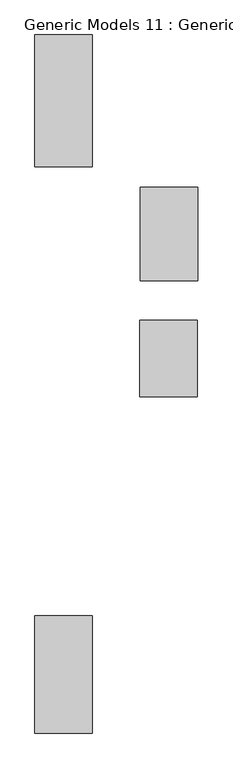
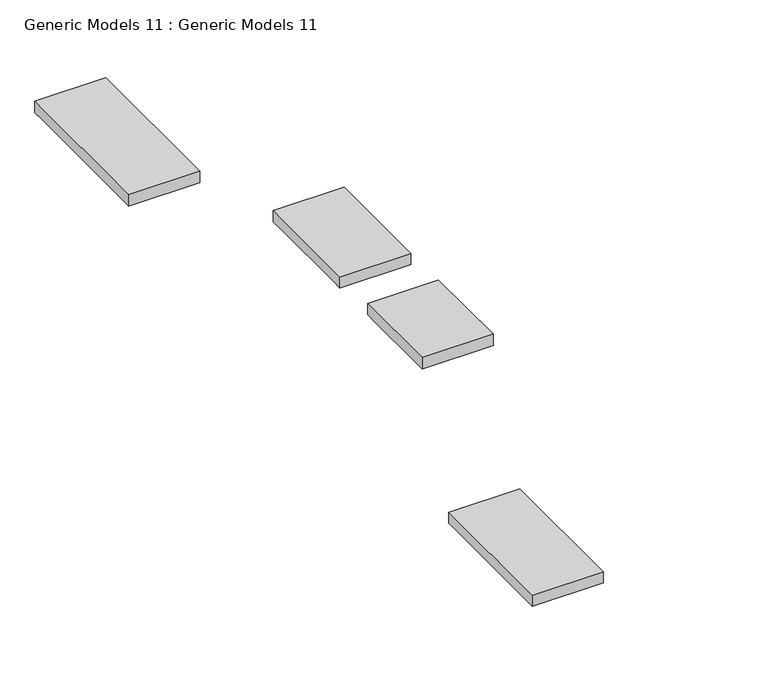
"""IFC4 building model written with IfcOpenShell, lengths in millimetres: proxy geometry, Generic Models 11 : Generic Models 11."""

from ifc_helpers import new_model, si_unit, frame, origin, place, context, project, spatial, polyline, outline, extrude, source, transform, mapped, element, save


def generic_models_11_generic_models_11_73ad1d2d(model_context):
    return source(origin(), model_context, "Body", "SweptSolid", [
        extrude(outline(polyline([(8100.454021, 5848.35), (7948.054021, 5848.35), (6385.954021, 5848.35), (6233.554021, 5848.35), (6233.554021, 6000.75), (8100.454021, 6000.75), (8100.454021, 5848.35)])), frame((-43007.0645004, 0.0, 0.0), z_axis=(1.0, 0.0, 0.0), x_axis=(0.0, 1.0, 0.0)), (0.0, 0.0, 1.0), 914.4),
        extrude(outline(polyline([(11586.604021, 5257.8), (11586.604021, 5410.2), (12805.804021, 5410.2), (12805.804021, 5257.8), (12653.404021, 5257.8), (11739.004021, 5257.8), (11586.604021, 5257.8)])), frame((-41337.0145004, 0.0, 0.0), z_axis=(1.0, 0.0, 0.0), x_axis=(0.0, 1.0, 0.0)), (0.0, 0.0, 1.0), 914.4),
        extrude(outline(polyline([(13434.454021, 5238.75), (13434.454021, 5391.15), (14920.354021, 5391.15), (14920.354021, 5238.75), (14767.954021, 5238.75), (13586.854021, 5238.75), (13434.454021, 5238.75)])), frame((-41330.6645004, 0.0, 0.0), z_axis=(1.0, 0.0, 0.0), x_axis=(0.0, 1.0, 0.0)), (0.0, 0.0, 1.0), 914.4),
        extrude(outline(polyline([(17346.054021, 5848.35), (17193.654021, 5848.35), (15244.1504636, 5848.35), (15244.1504636, 6000.75), (17346.054021, 6000.75), (17346.054021, 5848.35)])), frame((-43007.0645004, 0.0, 0.0), z_axis=(1.0, 0.0, 0.0), x_axis=(0.0, 1.0, 0.0)), (0.0, 0.0, 1.0), 914.4),
    ])


if __name__ == "__main__":
    model = new_model("IFC4")
    model_context = context("Model", 3, world=origin())
    ifc_project = project(units=[si_unit("LENGTHUNIT", "METRE", prefix="MILLI")], contexts=[model_context])
    site = spatial("IfcSite", under=ifc_project)
    building = spatial("IfcBuilding", under=site)
    placement = place(None, origin())
    generic_models_11_generic_models_11_shape = generic_models_11_generic_models_11_73ad1d2d(model_context)
    element("IfcBuildingElementProxy", 1, Name="Generic Models 11 : Generic Models 11", ObjectType="Generic Models 11 : Generic Models 11", at=placement, inside=building, context=model_context, shape_type="MappedRepresentation", body=[
        mapped(generic_models_11_generic_models_11_shape, transform((0.0, 0.0, 0.0), x_axis=(1.0, 0.0, 0.0), y_axis=(0.0, 1.0, 0.0), z_axis=(0.0, 0.0, 1.0))),
    ])
    save(model, "model.ifc")
